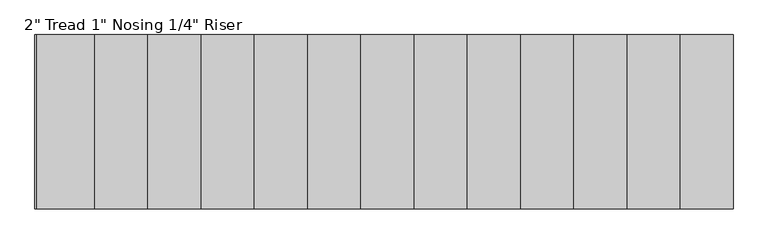
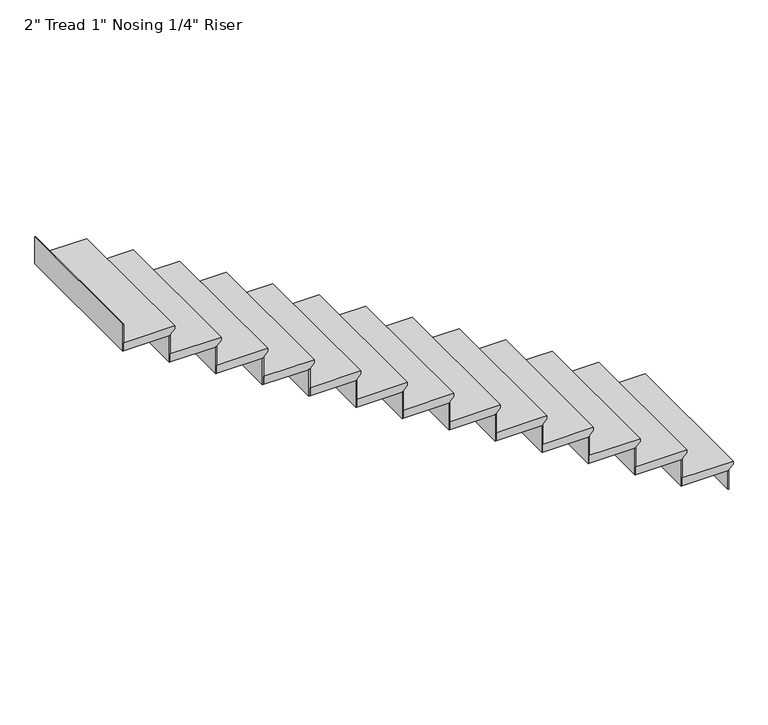
"""IFC4 building model written with IfcOpenShell, lengths in millimetres: stair flight geometry."""

from ifc_helpers import new_model, si_unit, frame, origin, place, context, project, spatial, polyline, outline, extrude, source, transform, mapped, element, save


def stair_flight_159ea243(model_context):
    return source(origin(), model_context, "Body", "SweptSolid", [
        extrude(outline(polyline([(338.6666667, -2390.4214984), (338.6666667, -2695.2214984), (287.8666667, -2695.2214984), (287.8666667, -2415.8214984), (294.2166667, -2415.8214984), (319.6166667, -2390.4214984), (338.6666667, -2390.4214984)])), frame((0.0, 4382.4166905, 0.0), z_axis=(0.0, 1.0, 0.0), x_axis=(0.0, 0.0, 1.0)), (0.0, 0.0, 1.0), 914.4),
        extrude(outline(polyline([(-2422.1714984, 5296.8166905), (-2415.8214984, 5296.8166905), (-2415.8214984, 4382.4166905), (-2422.1714984, 4382.4166905), (-2422.1714984, 5296.8166905)])), frame((0.0, 0.0, 169.3333333), z_axis=(0.0, 0.0, 1.0), x_axis=(1.0, 0.0, 0.0)), (0.0, 0.0, 1.0), 118.5333333),
        extrude(outline(polyline([(-2701.5714984, 5296.8166905), (-2695.2214984, 5296.8166905), (-2695.2214984, 4382.4166905), (-2701.5714984, 4382.4166905), (-2701.5714984, 5296.8166905)])), frame((0.0, 0.0, 287.8666667), z_axis=(0.0, 0.0, 1.0), x_axis=(1.0, 0.0, 0.0)), (0.0, 0.0, 1.0), 169.3333333),
        extrude(outline(polyline([(508.0, -2669.8214984), (508.0, -2974.6214984), (457.2, -2974.6214984), (457.2, -2695.2214984), (463.55, -2695.2214984), (488.95, -2669.8214984), (508.0, -2669.8214984)])), frame((0.0, 4382.4166905, 0.0), z_axis=(0.0, 1.0, 0.0), x_axis=(0.0, 0.0, 1.0)), (0.0, 0.0, 1.0), 914.4),
        extrude(outline(polyline([(-2980.9714984, 5296.8166905), (-2974.6214984, 5296.8166905), (-2974.6214984, 4382.4166905), (-2980.9714984, 4382.4166905), (-2980.9714984, 5296.8166905)])), frame((0.0, 0.0, 457.2), z_axis=(0.0, 0.0, 1.0), x_axis=(1.0, 0.0, 0.0)), (0.0, 0.0, 1.0), 169.3333333),
        extrude(outline(polyline([(677.3333333, -2949.2214984), (677.3333333, -3254.0214984), (626.5333333, -3254.0214984), (626.5333333, -2974.6214984), (632.8833333, -2974.6214984), (658.2833333, -2949.2214984), (677.3333333, -2949.2214984)])), frame((0.0, 4382.4166905, 0.0), z_axis=(0.0, 1.0, 0.0), x_axis=(0.0, 0.0, 1.0)), (0.0, 0.0, 1.0), 914.4),
        extrude(outline(polyline([(-3260.3714984, 5296.8166905), (-3254.0214984, 5296.8166905), (-3254.0214984, 4382.4166905), (-3260.3714984, 4382.4166905), (-3260.3714984, 5296.8166905)])), frame((0.0, 0.0, 626.5333333), z_axis=(0.0, 0.0, 1.0), x_axis=(1.0, 0.0, 0.0)), (0.0, 0.0, 1.0), 169.3333333),
        extrude(outline(polyline([(846.6666667, -3228.6214984), (846.6666667, -3533.4214984), (795.8666667, -3533.4214984), (795.8666667, -3254.0214984), (802.2166667, -3254.0214984), (827.6166667, -3228.6214984), (846.6666667, -3228.6214984)])), frame((0.0, 4382.4166905, 0.0), z_axis=(0.0, 1.0, 0.0), x_axis=(0.0, 0.0, 1.0)), (0.0, 0.0, 1.0), 914.4),
        extrude(outline(polyline([(-3539.7714984, 5296.8166905), (-3533.4214984, 5296.8166905), (-3533.4214984, 4382.4166905), (-3539.7714984, 4382.4166905), (-3539.7714984, 5296.8166905)])), frame((0.0, 0.0, 795.8666667), z_axis=(0.0, 0.0, 1.0), x_axis=(1.0, 0.0, 0.0)), (0.0, 0.0, 1.0), 169.3333333),
        extrude(outline(polyline([(1016.0, -3508.0214984), (1016.0, -3812.8214984), (965.2, -3812.8214984), (965.2, -3533.4214984), (971.55, -3533.4214984), (996.95, -3508.0214984), (1016.0, -3508.0214984)])), frame((0.0, 4382.4166905, 0.0), z_axis=(0.0, 1.0, 0.0), x_axis=(0.0, 0.0, 1.0)), (0.0, 0.0, 1.0), 914.4),
        extrude(outline(polyline([(-3819.1714984, 5296.8166905), (-3812.8214984, 5296.8166905), (-3812.8214984, 4382.4166905), (-3819.1714984, 4382.4166905), (-3819.1714984, 5296.8166905)])), frame((0.0, 0.0, 965.2), z_axis=(0.0, 0.0, 1.0), x_axis=(1.0, 0.0, 0.0)), (0.0, 0.0, 1.0), 169.3333333),
        extrude(outline(polyline([(1185.3333333, -3787.4214984), (1185.3333333, -4092.2214984), (1134.5333333, -4092.2214984), (1134.5333333, -3812.8214984), (1140.8833333, -3812.8214984), (1166.2833333, -3787.4214984), (1185.3333333, -3787.4214984)])), frame((0.0, 4382.4166905, 0.0), z_axis=(0.0, 1.0, 0.0), x_axis=(0.0, 0.0, 1.0)), (0.0, 0.0, 1.0), 914.4),
        extrude(outline(polyline([(-4098.5714984, 5296.8166905), (-4092.2214984, 5296.8166905), (-4092.2214984, 4382.4166905), (-4098.5714984, 4382.4166905), (-4098.5714984, 5296.8166905)])), frame((0.0, 0.0, 1134.5333333), z_axis=(0.0, 0.0, 1.0), x_axis=(1.0, 0.0, 0.0)), (0.0, 0.0, 1.0), 169.3333333),
        extrude(outline(polyline([(1354.6666667, -4066.8214984), (1354.6666667, -4371.6214984), (1303.8666667, -4371.6214984), (1303.8666667, -4092.2214984), (1310.2166667, -4092.2214984), (1335.6166667, -4066.8214984), (1354.6666667, -4066.8214984)])), frame((0.0, 4382.4166905, 0.0), z_axis=(0.0, 1.0, 0.0), x_axis=(0.0, 0.0, 1.0)), (0.0, 0.0, 1.0), 914.4),
        extrude(outline(polyline([(-4377.9714984, 5296.8166905), (-4371.6214984, 5296.8166905), (-4371.6214984, 4382.4166905), (-4377.9714984, 4382.4166905), (-4377.9714984, 5296.8166905)])), frame((0.0, 0.0, 1303.8666667), z_axis=(0.0, 0.0, 1.0), x_axis=(1.0, 0.0, 0.0)), (0.0, 0.0, 1.0), 169.3333333),
        extrude(outline(polyline([(1524.0, -4346.2214984), (1524.0, -4651.0214984), (1473.2, -4651.0214984), (1473.2, -4371.6214984), (1479.55, -4371.6214984), (1504.95, -4346.2214984), (1524.0, -4346.2214984)])), frame((0.0, 4382.4166905, 0.0), z_axis=(0.0, 1.0, 0.0), x_axis=(0.0, 0.0, 1.0)), (0.0, 0.0, 1.0), 914.4),
        extrude(outline(polyline([(-4657.3714984, 5296.8166905), (-4651.0214984, 5296.8166905), (-4651.0214984, 4382.4166905), (-4657.3714984, 4382.4166905), (-4657.3714984, 5296.8166905)])), frame((0.0, 0.0, 1473.2), z_axis=(0.0, 0.0, 1.0), x_axis=(1.0, 0.0, 0.0)), (0.0, 0.0, 1.0), 169.3333333),
        extrude(outline(polyline([(1693.3333333, -4625.6214984), (1693.3333333, -4930.4214984), (1642.5333333, -4930.4214984), (1642.5333333, -4651.0214984), (1648.8833333, -4651.0214984), (1674.2833333, -4625.6214984), (1693.3333333, -4625.6214984)])), frame((0.0, 4382.4166905, 0.0), z_axis=(0.0, 1.0, 0.0), x_axis=(0.0, 0.0, 1.0)), (0.0, 0.0, 1.0), 914.4),
        extrude(outline(polyline([(-4936.7714984, 5296.8166905), (-4930.4214984, 5296.8166905), (-4930.4214984, 4382.4166905), (-4936.7714984, 4382.4166905), (-4936.7714984, 5296.8166905)])), frame((0.0, 0.0, 1642.5333333), z_axis=(0.0, 0.0, 1.0), x_axis=(1.0, 0.0, 0.0)), (0.0, 0.0, 1.0), 169.3333333),
        extrude(outline(polyline([(1862.6666667, -4905.0214984), (1862.6666667, -5209.8214984), (1811.8666667, -5209.8214984), (1811.8666667, -4930.4214984), (1818.2166667, -4930.4214984), (1843.6166667, -4905.0214984), (1862.6666667, -4905.0214984)])), frame((0.0, 4382.4166905, 0.0), z_axis=(0.0, 1.0, 0.0), x_axis=(0.0, 0.0, 1.0)), (0.0, 0.0, 1.0), 914.4),
        extrude(outline(polyline([(-5216.1714984, 5296.8166905), (-5209.8214984, 5296.8166905), (-5209.8214984, 4382.4166905), (-5216.1714984, 4382.4166905), (-5216.1714984, 5296.8166905)])), frame((0.0, 0.0, 1811.8666667), z_axis=(0.0, 0.0, 1.0), x_axis=(1.0, 0.0, 0.0)), (0.0, 0.0, 1.0), 169.3333333),
        extrude(outline(polyline([(2032.0, -5184.4214984), (2032.0, -5489.2214984), (1981.2, -5489.2214984), (1981.2, -5209.8214984), (1987.55, -5209.8214984), (2012.95, -5184.4214984), (2032.0, -5184.4214984)])), frame((0.0, 4382.4166905, 0.0), z_axis=(0.0, 1.0, 0.0), x_axis=(0.0, 0.0, 1.0)), (0.0, 0.0, 1.0), 914.4),
        extrude(outline(polyline([(-5495.5714984, 5296.8166905), (-5489.2214984, 5296.8166905), (-5489.2214984, 4382.4166905), (-5495.5714984, 4382.4166905), (-5495.5714984, 5296.8166905)])), frame((0.0, 0.0, 1981.2), z_axis=(0.0, 0.0, 1.0), x_axis=(1.0, 0.0, 0.0)), (0.0, 0.0, 1.0), 169.3333333),
        extrude(outline(polyline([(2201.3333333, -5463.8214984), (2201.3333333, -5768.6214984), (2150.5333333, -5768.6214984), (2150.5333333, -5489.2214984), (2156.8833333, -5489.2214984), (2182.2833333, -5463.8214984), (2201.3333333, -5463.8214984)])), frame((0.0, 4382.4166905, 0.0), z_axis=(0.0, 1.0, 0.0), x_axis=(0.0, 0.0, 1.0)), (0.0, 0.0, 1.0), 914.4),
        extrude(outline(polyline([(-5774.9714984, 5296.8166905), (-5768.6214984, 5296.8166905), (-5768.6214984, 4382.4166905), (-5774.9714984, 4382.4166905), (-5774.9714984, 5296.8166905)])), frame((0.0, 0.0, 2150.5333333), z_axis=(0.0, 0.0, 1.0), x_axis=(1.0, 0.0, 0.0)), (0.0, 0.0, 1.0), 169.3333333),
        extrude(outline(polyline([(2370.6666667, -5743.2214984), (2370.6666667, -6048.0214984), (2319.8666667, -6048.0214984), (2319.8666667, -5768.6214984), (2326.2166667, -5768.6214984), (2351.6166667, -5743.2214984), (2370.6666667, -5743.2214984)])), frame((0.0, 4382.4166905, 0.0), z_axis=(0.0, 1.0, 0.0), x_axis=(0.0, 0.0, 1.0)), (0.0, 0.0, 1.0), 914.4),
        extrude(outline(polyline([(-6054.3714984, 5296.8166905), (-6048.0214984, 5296.8166905), (-6048.0214984, 4382.4166905), (-6054.3714984, 4382.4166905), (-6054.3714984, 5296.8166905)])), frame((0.0, 0.0, 2319.8666667), z_axis=(0.0, 0.0, 1.0), x_axis=(1.0, 0.0, 0.0)), (0.0, 0.0, 1.0), 169.3333333),
    ])


if __name__ == "__main__":
    model = new_model("IFC4")
    model_context = context("Model", 3, world=origin())
    ifc_project = project(units=[si_unit("LENGTHUNIT", "METRE", prefix="MILLI")], contexts=[model_context])
    site = spatial("IfcSite", under=ifc_project)
    building = spatial("IfcBuilding", under=site)
    placement = place(None, origin())
    stair_flight_shape = stair_flight_159ea243(model_context)
    element("IfcStairFlight", 1, ObjectType="2\" Tread 1\" Nosing 1/4\" Riser", at=placement, inside=building, context=model_context, shape_type="MappedRepresentation", body=[
        mapped(stair_flight_shape, transform((0.0, 0.0, 0.0), x_axis=(1.0, 0.0, 0.0), y_axis=(0.0, 1.0, 0.0), z_axis=(0.0, 0.0, 1.0))),
    ])
    save(model, "model.ifc")
